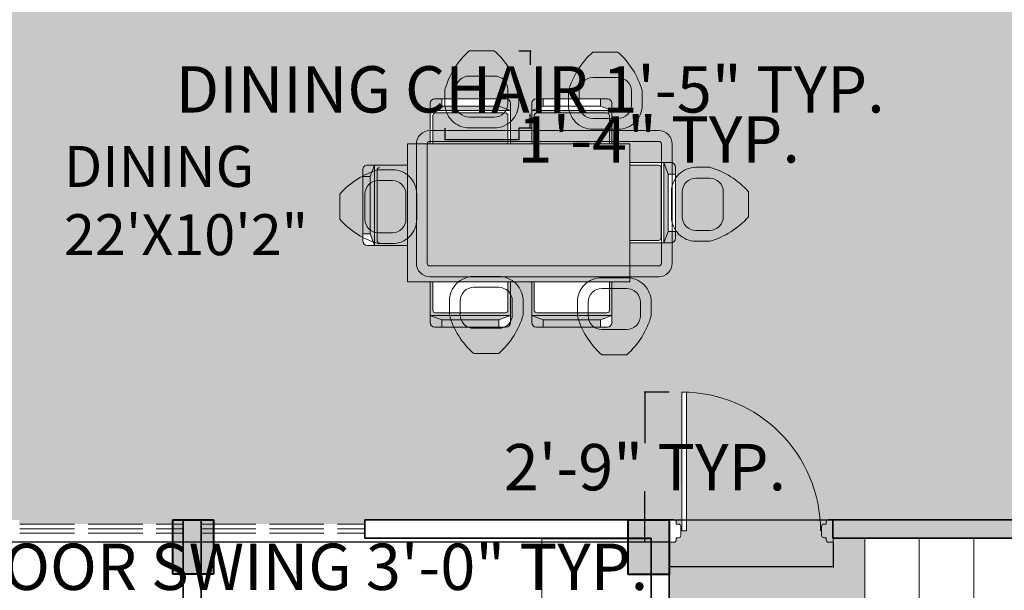
# Model space of a CAD drawing. Units: inches. Extents: x 1077 to 2505, y 1892 to 2728.
# Tile 23 of 26: x 2147 to 2364, y 2298 to 2423. Entities that reach past the tile are written whole.
import ezdxf

# ---------------------------------------------------------------- set-up
doc = ezdxf.new("R2010")
doc.units = ezdxf.units.IN
doc.linetypes.add('ACAD_ISO02W100', pattern=[15, 12, -3])
doc.layers.get('Defpoints').update_dxf_attribs({"color": 220, "linetype": 'ACAD_ISO02W100'})
for name, color, linetype, lineweight in [('00 FURNITURE', 15, 'Continuous', 15), ('A-ANNO-DIMS', 2, 'Continuous', 18), ('A-AREA-IDEN', 7, 'Continuous', 18), ('A-COLS', 7, 'Continuous', 40), ('A-DOOR', 4, 'Continuous', 18), ('A-FLOR-CASE', 8, 'Continuous', 18), ('A-FLOR-STRS', 7, 'Continuous', 18), ('A-GLAZ-OVHD', 160, 'ACAD_ISO02W100', 13), ('A-WALL-PATT', 7, 'Continuous', 9), ('WALL', 7, 'Continuous', 35)]:
    doc.layers.add(name, color=color, linetype=linetype, lineweight=lineweight)
doc.layers.add('A-FLOR-PATT', color=254, linetype='Continuous', lineweight=9, true_color=0xd7ebd2)
doc.styles.get("Standard").update_dxf_attribs({"font": 'arial.ttf'})
doc.dimstyles.get("Standard").update_dxf_attribs({"dimtxt": 10.18, "dimasz": 0.18, "dimexe": 0.18, "dimexo": 0.0625, "dimgap": 0.09, "dimtad": 0, "dimtih": 1, "dimtoh": 1, "dimdec": 0, "dimzin": 0, "dimdsep": 46, "dimlunit": 3, "dimtxsty": 'Standard', "dimcen": 0.09, "dimadec": 0, "dimazin": 0, "dimtfac": 1, "dimtdec": 0, "dimtofl": 0, "dimtmove": 0, "dimatfit": 3, "dimfxl": 1, "dimtolj": 1, "dimtzin": 0, "dimarcsym": 0})

# ---------------------------------------------------------------- blocks, each defined once
blk = doc.blocks.new('DDD')
at = {"layer": '00 FURNITURE'}
for p, q in [((-12579.77, -15859.53), (-12579.77, -15829.05)), ((-12578.77, -15859.53), (-12578.77, -15829.03)), ((-12612.02, -15857.03), (-12612.02, -15862.03)), ((-12611.02, -15857.03), (-12612.02, -15857.03)), ((-12610.52, -15858.03), (-12610.52, -15857.53)), ((-12577.52, -15858.03), (-12577.52, -15857.53)), ((-12577.02, -15857.03), (-12576.02, -15857.03)), ((-12576.02, -15857.03), (-12576.02, -15862.03)), ((-12578.77, -15859.53), (-12579.77, -15859.53)), ((-12612.02, -15862.03), (-12611.02, -15862.03)), ((-12610.52, -15861.53), (-12610.52, -15861.03)), ((-12577.52, -15861.53), (-12577.52, -15861.03)), ((-12576.02, -15862.03), (-12577.02, -15862.03))]:
    blk.add_line(p, q, dxfattribs=at)
for points in [[(-12610.52, -15861.03), (-12610.02, -15861.03, 0.414214), (-12609.52, -15860.53), (-12609.52, -15858.53, 0.414214), (-12610.02, -15858.03), (-12610.52, -15858.03)], [(-12577.52, -15861.03), (-12578.02, -15861.03, -0.414214), (-12578.52, -15860.53), (-12578.52, -15858.53, -0.414214), (-12578.02, -15858.03), (-12577.52, -15858.03)]]:
    blk.add_lwpolyline(points, format="xyb", dxfattribs=at)
for centre, radius, start, end in [((-12578.77, -15859.53), 30.5, 90, 180), ((-12611.02, -15857.53), 0.5, 0, 90), ((-12577.02, -15857.53), 0.5, 90, 180), ((-12611.02, -15861.53), 0.5, 270, 0), ((-12577.02, -15861.53), 0.5, 180, 270)]:
    blk.add_arc(centre, radius, start, end, dxfattribs=at)
blk = doc.blocks.new('C1')
h = blk.add_hatch(color=256)
h.dxf.hatch_style = 1
h.paths.add_polyline_path([(1668.56, 2445.41), (1677.56, 2445.41), (1677.56, 2457.41), (1668.56, 2457.41)])
for p, q in [((1668.56, 2457.41), (1677.56, 2457.41)), ((1668.56, 2445.41), (1668.56, 2457.41)), ((1677.56, 2457.41), (1677.56, 2445.41)), ((1677.56, 2445.41), (1668.56, 2445.41))]:
    blk.add_line(p, q)
blk = doc.blocks.new('DINING-SET-6-SEAT')
for p, q in [((15.87, 50.2), (31.49, 50.2)), ((38.2, 50.2), (53.82, 50.2)), ((14.85, 40.27), (14.85, 49.18)), ((17.38, 48.59), (14.85, 47.63)), ((17.38, 48.59), (29.95, 48.59)), ((29.95, 48.59), (32.51, 47.63)), ((32.51, 49.18), (32.51, 40.27)), ((37.18, 40.27), (37.18, 49.18)), ((39.7, 48.59), (37.18, 47.63)), ((39.7, 48.59), (52.28, 48.59)), ((52.28, 48.59), (54.83, 47.63)), ((54.83, 49.18), (54.83, 40.27)), ((14.85, 47.63), (32.51, 47.63)), ((15.41, 40.27), (15.41, 46.51)), ((15.97, 47.07), (31.38, 47.07)), ((31.94, 46.51), (31.94, 40.27)), ((37.18, 47.63), (54.83, 47.63)), ((37.74, 40.27), (37.74, 46.51)), ((38.3, 47.07), (53.71, 47.07)), ((54.27, 46.51), (54.27, 40.27)), ((58.75, 40.27), (9.82, 40.27)), ((9.82, 9.93), (9.82, 40.27)), ((58.75, 9.93), (58.75, 40.27)), ((9.93, 35.61), (1.02, 35.61)), ((1.62, 33.08), (2.57, 35.61)), ((2.57, 35.61), (2.57, 17.96)), ((58.86, 36.15), (67.76, 36.15)), ((58.86, 35.58), (65.09, 35.58)), ((65.65, 35.02), (65.65, 19.61)), ((67.17, 33.62), (66.22, 36.15)), ((66.22, 36.15), (66.22, 18.49)), ((68.78, 35.13), (68.78, 19.51)), ((0, 34.59), (0, 18.97)), ((1.62, 33.08), (1.62, 20.51)), ((3.13, 34.49), (3.13, 19.08)), ((67.17, 33.62), (67.17, 21.04)), ((1.62, 20.51), (2.57, 17.96)), ((67.17, 21.04), (66.22, 18.49)), ((1.02, 17.96), (9.93, 17.96)), ((65.09, 19.05), (58.86, 19.05)), ((67.76, 18.49), (58.86, 18.49)), ((58.75, 9.93), (9.82, 9.93)), ((14.85, 9.93), (14.85, 1.02)), ((15.41, 9.93), (15.41, 3.69)), ((31.94, 3.69), (31.94, 9.93)), ((32.51, 1.02), (32.51, 9.93)), ((37.18, 9.93), (37.18, 1.02)), ((37.74, 9.93), (37.74, 3.69)), ((54.27, 3.69), (54.27, 9.93)), ((54.83, 1.02), (54.83, 9.93)), ((17.38, 1.61), (14.85, 2.57)), ((14.85, 2.57), (32.51, 2.57)), ((15.97, 3.13), (31.38, 3.13)), ((29.95, 1.61), (32.51, 2.57)), ((39.7, 1.61), (37.18, 2.57)), ((37.18, 2.57), (54.83, 2.57)), ((38.3, 3.13), (53.71, 3.13)), ((52.28, 1.61), (54.83, 2.57)), ((17.38, 1.61), (29.95, 1.61)), ((39.7, 1.61), (52.28, 1.61)), ((15.87, 0), (31.49, 0)), ((38.2, 0), (53.82, 0))]:
    blk.add_line(p, q)
for points in [[(17.38, 50.2), (29.95, 50.2), (29.95, 48.59), (17.38, 48.59)], [(39.7, 50.2), (52.28, 50.2), (52.28, 48.59), (39.7, 48.59)], [(0, 33.08), (0, 20.51), (1.62, 20.51), (1.62, 33.08)], [(68.78, 33.62), (68.78, 21.04), (67.17, 21.04), (67.17, 33.62)], [(17.38, 0), (29.95, 0), (29.95, 1.61), (17.38, 1.61)], [(39.7, 0), (52.28, 0), (52.28, 1.61), (39.7, 1.61)]]:
    blk.add_lwpolyline(points, close=True)
for centre, radius, start, end in [((15.87, 49.18), 1.02, 90.0001, 180.0001), ((31.49, 49.18), 1.02, 0.0001, 90.0001), ((38.2, 49.18), 1.02, 90.0001, 180.0001), ((53.82, 49.18), 1.02, 0.0001, 90.0001), ((15.97, 46.51), 0.56, 90.0001, 180.0001), ((31.38, 46.51), 0.56, 0.0001, 90.0001), ((38.3, 46.51), 0.56, 90.0001, 180.0001), ((53.71, 46.51), 0.56, 0.0001, 90.0001), ((1.02, 34.59), 1.02, 89.9999, 179.9999), ((3.69, 34.49), 0.56, 89.9999, 179.9999), ((65.09, 35.02), 0.56, 0.0001, 90.0001), ((67.76, 35.13), 1.02, 0.0001, 90.0001), ((65.09, 19.61), 0.56, 270.0001, 0.0001), ((67.76, 19.51), 1.02, 270.0001, 0.0001), ((1.02, 18.97), 1.02, 179.9999, 269.9999), ((3.69, 19.08), 0.56, 179.9999, 269.9999), ((15.97, 3.69), 0.56, 179.9999, 269.9999), ((31.38, 3.69), 0.56, 269.9999, 359.9999), ((38.3, 3.69), 0.56, 179.9999, 269.9999), ((53.71, 3.69), 0.56, 269.9999, 359.9999), ((15.87, 1.02), 1.02, 179.9999, 269.9999), ((31.49, 1.02), 1.02, 269.9999, 359.9999), ((38.2, 1.02), 1.02, 179.9999, 269.9999), ((53.82, 1.02), 1.02, 269.9999, 359.9999)]:
    blk.add_arc(centre, radius, start, end)
blk = doc.blocks.new('DINING-CHAIR')
for points in [[(5.36, 16.93), (10.88, 16.93, -0.142909), (16.24, 8.42), (16.24, 5.36, -0.414214), (10.88, 0), (5.36, 0, -0.414214), (0, 5.36), (0, 8.42, -0.142909)], [(5.36, 11.39), (10.88, 11.39, -0.414214), (13.86, 8.42), (13.86, 5.36, -0.414214), (10.88, 2.38), (5.36, 2.38, -0.414214), (2.38, 5.36), (2.38, 8.42, -0.414214)]]:
    blk.add_lwpolyline(points, format="xyb", close=True)
blk = doc.blocks.new('STAIR-PLAN-RETURN')
for p, q in [((0, 163.08), (0, 127.08)), ((12, 163.08), (12, 127.08)), ((24, 163.08), (24, 127.08)), ((36, 163.08), (36, 0)), ((36, 163.08), (36, 127.08)), ((0, 127.08), (72, 127.08)), ((36, 115.08), (72, 115.08)), ((36, 103.08), (72, 103.08)), ((36, 91.08), (72, 91.08)), ((36, 79.08), (72, 79.08)), ((36, 67.08), (72, 67.08)), ((36, 55.08), (72, 55.08)), ((36, 43.08), (72, 43.08)), ((36, 31.08), (72, 31.08)), ((36, 19.08), (72, 19.08)), ((36, 7.08), (72, 7.08)), ((72, 0), (36, 0))]:
    blk.add_line(p, q)
blk = doc.blocks.new('*D46')
at = {"layer": 'A-ANNO-DIMS', "color": 0, "lineweight": -2, "transparency": 16777216}
for p, q in [((2289.89, 2308.17), (2289.89, 2302.65)), ((2325.89, 2308.17), (2325.89, 2302.65)), ((2289.89, 2302.83), (2289.71, 2302.83)), ((2325.71, 2302.83), (2290.07, 2302.83))]:
    blk.add_line(p, q, dxfattribs=at)
at = {"layer": 'A-ANNO-DIMS', "color": 0, "transparency": 16777216}
for points in [[(2290.07, 2302.86), (2290.07, 2302.8), (2289.89, 2302.83)], [(2325.71, 2302.86), (2325.71, 2302.8), (2325.89, 2302.83)]]:
    blk.add_solid(points, dxfattribs=at)
at = {"layer": 'Defpoints', "color": 0, "transparency": 16777216}
for p in [(2289.89, 2308.23), (2325.89, 2308.23), (2289.89, 2302.83)]:
    blk.add_point(p, dxfattribs=at)
at = {"layer": 'A-ANNO-DIMS', "color": 0, "transparency": 16777216, "insert": (2209.47, 2302.83), "char_height": 10.18, "attachment_point": 5}
blk.add_mtext('\\A1;DOOR SWING 3\'-0" TYP.', dxfattribs=at)
blk = doc.blocks.new('*D47')
at = {"layer": 'A-ANNO-DIMS', "color": 0, "lineweight": -2, "transparency": 16777216}
for p, q in [((2289.82, 2341.23), (2284.31, 2341.23)), ((2284.49, 2341.05), (2284.49, 2330.02)), ((2284.49, 2308.41), (2284.49, 2319.44)), ((2289.82, 2308.23), (2284.31, 2308.23))]:
    blk.add_line(p, q, dxfattribs=at)
at = {"layer": 'A-ANNO-DIMS', "color": 0, "transparency": 16777216}
for points in [[(2284.46, 2341.05), (2284.52, 2341.05), (2284.49, 2341.23)], [(2284.46, 2308.41), (2284.52, 2308.41), (2284.49, 2308.23)]]:
    blk.add_solid(points, dxfattribs=at)
at = {"layer": 'Defpoints', "color": 0, "transparency": 16777216}
for p in [(2284.49, 2341.23), (2289.89, 2341.23), (2289.89, 2308.23)]:
    blk.add_point(p, dxfattribs=at)
at = {"layer": 'A-ANNO-DIMS', "color": 0, "transparency": 16777216, "insert": (2284.49, 2324.73), "char_height": 10.18, "attachment_point": 5}
blk.add_mtext('\\A1;2\'-9" TYP.', dxfattribs=at)
blk = doc.blocks.new('*D48')
at = {"layer": 'A-ANNO-DIMS', "color": 0, "lineweight": -2, "transparency": 16777216}
for p, q in [((2256.78, 2416.24), (2259.43, 2416.24)), ((2259.25, 2416.06), (2259.25, 2413.13)), ((2259.25, 2399.49), (2259.25, 2402.42)), ((2256.78, 2399.31), (2259.43, 2399.31))]:
    blk.add_line(p, q, dxfattribs=at)
at = {"layer": 'A-ANNO-DIMS', "color": 0, "transparency": 16777216}
for points in [[(2259.22, 2416.06), (2259.28, 2416.06), (2259.25, 2416.24)], [(2259.22, 2399.49), (2259.28, 2399.49), (2259.25, 2399.31)]]:
    blk.add_solid(points, dxfattribs=at)
at = {"layer": 'Defpoints', "color": 0, "transparency": 16777216}
for p in [(2256.72, 2416.24), (2259.25, 2416.24), (2256.72, 2399.31)]:
    blk.add_point(p, dxfattribs=at)
at = {"layer": 'A-ANNO-DIMS', "color": 0, "transparency": 16777216, "insert": (2259.25, 2407.77), "char_height": 10.18, "attachment_point": 5}
blk.add_mtext('\\A1;DINING CHAIR 1\'-5" TYP.', dxfattribs=at)
blk = doc.blocks.new('*D49')
at = {"layer": 'A-ANNO-DIMS', "color": 0, "lineweight": -2, "transparency": 16777216}
for p, q in [((2240.47, 2399.25), (2240.47, 2396.59)), ((2256.72, 2399.25), (2256.72, 2396.59)), ((2240.65, 2396.77), (2256.54, 2396.77)), ((2256.72, 2396.77), (2256.9, 2396.77))]:
    blk.add_line(p, q, dxfattribs=at)
at = {"layer": 'A-ANNO-DIMS', "color": 0, "transparency": 16777216}
for points in [[(2240.65, 2396.8), (2240.65, 2396.74), (2240.47, 2396.77)], [(2256.54, 2396.8), (2256.54, 2396.74), (2256.72, 2396.77)]]:
    blk.add_solid(points, dxfattribs=at)
at = {"layer": 'Defpoints', "color": 0, "transparency": 16777216}
for p in [(2240.47, 2399.31), (2256.72, 2399.31), (2256.72, 2396.77)]:
    blk.add_point(p, dxfattribs=at)
at = {"layer": 'A-ANNO-DIMS', "color": 0, "transparency": 16777216, "insert": (2287.53, 2396.77), "char_height": 10.18, "attachment_point": 5}
blk.add_mtext('\\A1;1\'-4" TYP.', dxfattribs=at)
blk = doc.blocks.new('*D68')
at = {"layer": 'A-ANNO-DIMS', "color": 0, "lineweight": -2, "transparency": 16777216}
for p, q in [((2289.82, 2308.23), (2006.75, 2308.23)), ((2006.93, 2308.05), (2006.93, 2206.47)), ((2006.93, 2094.32), (2006.93, 2195.9)), ((2289.78, 2094.14), (2006.75, 2094.14))]:
    blk.add_line(p, q, dxfattribs=at)
at = {"layer": 'A-ANNO-DIMS', "color": 0, "transparency": 16777216}
for points in [[(2006.9, 2308.05), (2006.96, 2308.05), (2006.93, 2308.23)], [(2006.9, 2094.32), (2006.96, 2094.32), (2006.93, 2094.14)]]:
    blk.add_solid(points, dxfattribs=at)
at = {"layer": 'Defpoints', "color": 0, "transparency": 16777216}
for p in [(2006.93, 2308.23), (2289.89, 2308.23), (2289.85, 2094.14)]:
    blk.add_point(p, dxfattribs=at)
at = {"layer": 'A-ANNO-DIMS', "color": 0, "transparency": 16777216, "insert": (2006.93, 2201.18), "char_height": 10.18, "attachment_point": 5}
blk.add_mtext('\\A1;17\'-10"', dxfattribs=at)
blk = doc.blocks.new('*D72')
at = {"layer": 'A-ANNO-DIMS', "color": 0, "lineweight": -2, "transparency": 16777216}
for p, q in [((2280.86, 2313.12), (2442.88, 2313.12)), ((2442.7, 2312.94), (2442.7, 2303.7)), ((2442.7, 2283.76), (2442.7, 2292.99)), ((2285.24, 2283.58), (2442.88, 2283.58))]:
    blk.add_line(p, q, dxfattribs=at)
at = {"layer": 'A-ANNO-DIMS', "color": 0, "transparency": 16777216}
for points in [[(2442.67, 2312.94), (2442.73, 2312.94), (2442.7, 2313.12)], [(2442.67, 2283.76), (2442.73, 2283.76), (2442.7, 2283.58)]]:
    blk.add_solid(points, dxfattribs=at)
at = {"layer": 'Defpoints', "color": 0, "transparency": 16777216}
for p in [(2280.8, 2313.12), (2285.18, 2283.58), (2442.7, 2283.58)]:
    blk.add_point(p, dxfattribs=at)
at = {"layer": 'A-ANNO-DIMS', "color": 0, "transparency": 16777216, "insert": (2442.7, 2298.35), "char_height": 10.18, "attachment_point": 5}
blk.add_mtext('\\A1;2\'-5 1/2"', dxfattribs=at)

msp = doc.modelspace()

# ---------------------------------------------------------------- hatches: boundary and pattern name
at = {"layer": 'A-FLOR-PATT', "transparency": 33554559}
h = msp.add_hatch(color=256, dxfattribs=at)
h.dxf.hatch_style = 1
h.paths.add_polyline_path([(2252.85, 2583.14), (2232.15, 2583.14), (2208.15, 2583.17), (2208.15, 2583.14), (2186.85, 2583.14), (2186.85, 2486.14), (2186.85, 2475.14), (2182.85, 2475.14), (2182.85, 2521.11), (2164.84, 2521.11), (2164.84, 2583.14), (2126.63, 2583.14), (2078.63, 2583.13), (2078.63, 2583.14), (2044.85, 2583.14), (2044.85, 2439.14), (2146.85, 2439.14), (2146.85, 2435.14), (2120.85, 2435.14), (2044.85, 2435.14), (2044.85, 2401), (2044.85, 2401), (2044.85, 2377), (2044.85, 2377), (2044.85, 2313.14), (2116.85, 2313.14), (2116.85, 2405.14), (2120.85, 2405.14), (2120.85, 2313.14), (2146.85, 2313.14), (2146.85, 2312.21), (2182.85, 2312.21), (2182.85, 2313.14), (2186.85, 2313.14), (2186.85, 2312.21), (2222.85, 2312.21), (2222.85, 2313.14), (2289.85, 2313.14), (2289.85, 2094.14), (2404.85, 2094.14), (2404.85, 2146.06), (2368.85, 2146.06), (2368.85, 2273.14), (2332.85, 2273.14), (2332.85, 2309.14), (2325.85, 2309.14), (2325.85, 2313.14), (2404.85, 2313.14), (2404.85, 2354.2), (2404.85, 2402.2), (2404.85, 2435.14), (2292.85, 2435.14), (2292.85, 2439.14), (2333.66, 2439.14), (2333.66, 2457.16), (2404.85, 2457.16), (2404.85, 2583.14), (2356.85, 2583.14), (2356.85, 2592.14), (2404.85, 2592.14), (2404.85, 2648.14), (2375.5, 2648.14), (2375.5, 2648.03), (2351.47, 2648.03), (2351.47, 2648.14), (2326.85, 2648.14), (2326.85, 2583.14), (2256.85, 2583.14), (2256.85, 2435.14), (2182.85, 2435.14), (2182.85, 2439.14), (2186.85, 2439.14), (2252.85, 2439.14), (2252.85, 2486.14), (2216.85, 2486.14), (2216.85, 2490.14), (2252.85, 2490.14)])
h.paths.add_polyline_path([(2214.97, 2488.05), (2212.97, 2488.05), (2212.97, 2487.05, 0.414214), (2213.97, 2486.05), (2201.97, 2486.05), (2201.97, 2483.04), (2200.58, 2483.04), (2200.58, 2486.05), (2187.97, 2486.05, -0.414214), (2186.97, 2487.05), (2186.97, 2490.05), (2188.97, 2490.05), (2188.97, 2516.05, -0.446908)], flags=16)
h.paths.add_polyline_path([(2162.4, 2565.16), (2146.2, 2565.16), (2146.2, 2581.36), (2162.4, 2581.36)], flags=16)
h.paths.add_polyline_path([(2161.5, 2566.06), (2147.1, 2566.06), (2147.1, 2580.46), (2161.5, 2580.46)], flags=0)
h.paths.add_polyline_path([(2145.3, 2506.66, -0.414214), (2144.4, 2505.76), (2122.45, 2505.76), (2081.4, 2505.76, -0.414214), (2080.5, 2506.66), (2080.5, 2563.14), (2080.5, 2577.72), (2080.5, 2581.36), (2145.3, 2581.36), (2145.3, 2577.72), (2144.4, 2577.72, -0.414214), (2145.3, 2576.82)], flags=16)
h.paths.add_polyline_path([(2150.3, 2575.03, -1), (2158.24, 2575.03, -1)], flags=0)
h.paths.add_polyline_path([(2150.64, 2575.03, -1), (2157.89, 2575.03, -1)], flags=0)
h.paths.add_polyline_path([(2180.11, 2468.19), (2180.11, 2437.69), (2180.36, 2436.69), (2180.36, 2437.69), (2179.11, 2437.69), (2179.11, 2468.17, 0.404641), (2149.61, 2437.69), (2149.36, 2436.69, -0.414214), (2148.86, 2436.19), (2148.36, 2436.19), (2148.36, 2435.69, -0.414214), (2147.86, 2435.19), (2146.86, 2435.19), (2146.86, 2440.19), (2147.86, 2440.19, -0.414214), (2148.36, 2439.69), (2148.36, 2439.19), (2148.86, 2439.19, -0.414214), (2149.36, 2438.69), (2149.61, 2437.69, -0.414214)], flags=16)
h.paths.add_polyline_path([(2145.14, 2554.26, 0.292232), (2136.49, 2542.78, 0.052719), (2081.25, 2554.26), (2080.6, 2554.26), (2080.6, 2563.14), (2081.25, 2563.14), (2102.73, 2563.14, -0.117785), (2103.09, 2563.91, -0.059418), (2112.19, 2573, -0.379859), (2114.6, 2572.86, -0.02509), (2118.73, 2569.3, -0.025935), (2122.97, 2573, -0.379859), (2125.38, 2572.86, -0.061767), (2134.84, 2563.41, -0.069393), (2135.14, 2563.14), (2145.14, 2563.14)], flags=0)
h.paths.add_polyline_path([(2120.79, 2554.26), (2117.88, 2554.26, -0.015371), (2115.33, 2552.11, -0.429576), (2112.69, 2552.04, -0.016036), (2110.01, 2554.26), (2080.6, 2554.26), (2080.6, 2560.4), (2104.1, 2560.4, 0.055344), (2112.69, 2552.04, 0.331768), (2114.84, 2551.72, 0.027343), (2119.32, 2555.62, 0.00919)], flags=0)
h.paths.add_polyline_path([(2152.88, 2574.32), (2154.19, 2575.07), (2154.19, 2576.58, 0.399698), (2152.71, 2575.03, 0.119004)], flags=0)
h.paths.add_polyline_path([(2152.53, 2575.03, -1), (2156, 2575.03, -1)], flags=0)
h.paths.add_polyline_path([(2154.27, 2574.94), (2154.34, 2574.98), (2154.34, 2575.07), (2154.3, 2575.09), (2154.23, 2574.96)], flags=0)
h.paths.add_polyline_path([(2259.6, 2468.17, -0.414214), (2290.1, 2437.67), (2290.35, 2438.67), (2290.1, 2437.67, 0.404641), (2260.6, 2468.15), (2260.6, 2437.67), (2259.35, 2437.67), (2259.35, 2436.67, -0.414214), (2258.85, 2436.17), (2258.35, 2436.17), (2258.35, 2435.67, -0.414214), (2257.85, 2435.17), (2256.85, 2435.17), (2256.85, 2440.17), (2257.85, 2440.17, -0.414214), (2258.35, 2439.67), (2258.35, 2439.17), (2258.85, 2439.17, -0.414214), (2259.35, 2438.67)], flags=16)
h.paths.add_polyline_path([(2327.48, 2541.19, -0.414214), (2328.38, 2542.09), (2384.85, 2542.09), (2399.43, 2542.09), (2403.08, 2542.09), (2403.08, 2477.29), (2399.43, 2477.29), (2399.43, 2478.19, -0.414214), (2398.53, 2477.29), (2328.38, 2477.29, -0.414214), (2327.48, 2478.19), (2327.48, 2500.14)], flags=16)
h.paths.add_polyline_path([(2340.38, 2542.09, 0.253465), (2337.43, 2532.13, 0.2538), (2327.47, 2529.17)], flags=16)
h.paths.add_polyline_path([(2080.5, 2518.67, 0.253465), (2090.46, 2515.72, 0.2538), (2093.42, 2505.75)], flags=16)
h.paths.add_polyline_path([(2327.09, 2584.7), (2327.09, 2587.7), (2329.09, 2587.7), (2329.09, 2613.7, -0.01951), (2331.09, 2613.66), (2331.09, 2585.7), (2331.09, 2584.7, -0.414214), (2330.09, 2583.7), (2328.09, 2583.7, -0.414214)], flags=16)
h.paths.add_polyline_path([(2239.78, 2404.11), (2252.36, 2404.11), (2252.36, 2405.72), (2239.78, 2405.72)], flags=16)
h.paths.add_polyline_path([(2237.26, 2403.16), (2237.26, 2395.8), (2237.82, 2395.8), (2237.82, 2402.03, -0.41429), (2238.38, 2402.59), (2253.79, 2402.59, -0.414213), (2254.35, 2402.03), (2254.35, 2395.8), (2254.91, 2395.8), (2254.91, 2403.16)], flags=16)
h.paths.add_polyline_path([(2120.69, 2434.12), (2120.69, 2432.12, -0.414214), (2119.69, 2431.12), (2118.69, 2431.12), (2090.73, 2431.12, 0.400854), (2116.69, 2407.02), (2116.69, 2407.12), (2118.69, 2407.12, -0.446908), (2090.69, 2433.12), (2116.69, 2433.12), (2116.69, 2435.12), (2119.69, 2435.12, -0.414214)], flags=16)
h.paths.add_polyline_path([(2262.11, 2404.11), (2274.69, 2404.11), (2274.69, 2405.72), (2262.11, 2405.72)], flags=16)
h.paths.add_polyline_path([(2259.59, 2403.16), (2262.11, 2404.11), (2274.69, 2404.11), (2277.24, 2403.16)], flags=16)
h.paths.add_polyline_path([(2289.58, 2389.14), (2289.58, 2376.57), (2291.19, 2376.57), (2291.19, 2389.14)], flags=16)
h.paths.add_polyline_path([(2288.62, 2391.67), (2281.15, 2391.67), (2281.15, 2391.11), (2287.5, 2391.11, -0.41429), (2288.06, 2390.54), (2288.06, 2375.14, -0.414237), (2287.5, 2374.58), (2281.15, 2374.58), (2281.15, 2374.01), (2288.62, 2374.01)], flags=16)
h.paths.add_polyline_path([(2274.69, 2357.14), (2274.69, 2355.52), (2276.22, 2355.52, 0.414236), (2277.24, 2356.54), (2277.24, 2358.09)], flags=16)
h.paths.add_polyline_path([(2252.36, 2357.14), (2252.36, 2355.52), (2253.89, 2355.52, 0.414235), (2254.91, 2356.54), (2254.91, 2358.09)], flags=16)
h.paths.add_polyline_path([(2224.02, 2376.03), (2222.41, 2376.03), (2222.41, 2374.5, 0.414235), (2223.43, 2373.48), (2224.98, 2373.48)], flags=16)
h.paths.add_polyline_path([(2276.68, 2365.45), (2276.68, 2359.22, -0.41419), (2276.12, 2358.66), (2260.71, 2358.66, -0.414137), (2260.15, 2359.22), (2260.15, 2365.45), (2254.35, 2365.45), (2254.35, 2359.22, -0.414189), (2253.79, 2358.66), (2238.38, 2358.66, -0.414137), (2237.82, 2359.22), (2237.82, 2365.45)], flags=16)
h.paths.add_polyline_path([(2079.6, 2565.16), (2063.4, 2565.16), (2063.4, 2581.36), (2079.6, 2581.36)], flags=16)
h.paths.add_polyline_path([(2078.7, 2566.06), (2064.3, 2566.06), (2064.3, 2580.46), (2078.7, 2580.46)], flags=0)
h.paths.add_polyline_path([(2339.31, 2583.7), (2339.31, 2586.71), (2340.7, 2586.71), (2340.7, 2583.7), (2342.09, 2583.7), (2342.09, 2580.7), (2340.7, 2580.7), (2340.7, 2583.7)], flags=16)
h.paths.add_polyline_path([(2123.69, 2421.51), (2123.69, 2420.12), (2120.69, 2420.12), (2120.69, 2421.51), (2117.68, 2421.51), (2117.68, 2422.89), (2120.69, 2422.89), (2120.69, 2421.51)], flags=16)
h.paths.add_polyline_path([(2067.57, 2575.03, -1), (2075.51, 2575.03, -1)], flags=0)
h.paths.add_polyline_path([(2067.92, 2575.03, -1), (2075.17, 2575.03, -1)], flags=0)
h.paths.add_polyline_path([(2070.16, 2574.32), (2071.47, 2575.07), (2071.47, 2576.58, 0.399698), (2069.99, 2575.03, 0.119004)], flags=0)
h.paths.add_polyline_path([(2069.81, 2575.03, -1), (2073.28, 2575.03, -1)], flags=0)
h.paths.add_polyline_path([(2071.54, 2574.94), (2071.62, 2574.89), (2071.62, 2574.98)], flags=0)
h.paths.add_polyline_path([(2364.5, 2486.1, 0.052719), (2375.98, 2541.34), (2375.98, 2541.99), (2384.85, 2541.99), (2384.85, 2541.34), (2384.85, 2519.86, -0.117785), (2385.62, 2519.51, -0.059418), (2394.72, 2510.41, -0.379859), (2394.58, 2507.99, -0.02509), (2391.01, 2503.87, -0.025935), (2394.72, 2499.62, -0.379859), (2394.58, 2497.21, -0.061767), (2385.12, 2487.75, -0.069393), (2384.85, 2487.45), (2384.85, 2477.45), (2375.98, 2477.45, 0.292232)], flags=0)
h.paths.add_polyline_path([(2373.75, 2509.9, -0.016036), (2375.98, 2512.58), (2375.98, 2541.99), (2382.12, 2541.99), (2382.12, 2518.49, 0.055344), (2373.75, 2509.9, 0.331768), (2373.44, 2507.75, 0.027343), (2377.33, 2503.27, 0.00919), (2375.98, 2501.8), (2375.98, 2504.71, -0.015371), (2373.82, 2507.26, -0.429576)], flags=0)
h.paths.add_polyline_path([(2356.95, 2631.48, -0.171636), (2360.13, 2636.99), (2360.13, 2639.35), (2356, 2639.35, -0.414214), (2355.01, 2640.34), (2355.01, 2646.64, -0.414214), (2356, 2647.62), (2372.14, 2647.62, -0.414214), (2373.13, 2646.64), (2373.13, 2640.34, -0.414214), (2372.14, 2639.35), (2368.01, 2639.35), (2368.01, 2636.99, -0.171636), (2371.2, 2631.48, -0.258205), (2366.63, 2620.45), (2361.51, 2620.45, -0.258205)], flags=16)
h.paths.add_polyline_path([(2358.52, 2631.48, -0.171636), (2361.71, 2636.99), (2366.43, 2636.99, -0.171636), (2369.62, 2631.48, -0.210384), (2366.67, 2622), (2361.47, 2622, -0.210384)], flags=0)
h.paths.add_polyline_path([(2386.88, 2542.99), (2386.88, 2559.19), (2403.08, 2559.19), (2403.08, 2542.99)], flags=16)
h.paths.add_polyline_path([(2387.78, 2543.89), (2387.78, 2558.29), (2402.18, 2558.29), (2402.18, 2543.89)], flags=0)
h.paths.add_polyline_path([(2392.77, 2551.05, -1), (2400.71, 2551.05, -1)], flags=0)
h.paths.add_polyline_path([(2393.11, 2551.05, -1), (2400.37, 2551.05, -1)], flags=0)
h.paths.add_polyline_path([(2386.88, 2476.39), (2403.08, 2476.39), (2403.08, 2460.19), (2386.88, 2460.19)], flags=16)
h.paths.add_polyline_path([(2398.48, 2550.97), (2398.3, 2550.97, -0.544606), (2396.03, 2549.66), (2395.94, 2549.51, 0.547962)], flags=0)
h.paths.add_polyline_path([(2387.78, 2475.49), (2402.18, 2475.49), (2402.18, 2461.09), (2387.78, 2461.09)], flags=0)
h.paths.add_polyline_path([(2396.79, 2551.12), (2396.74, 2551.2), (2396.7, 2551.12)], flags=0)
h.paths.add_polyline_path([(2400.71, 2468.32, -1), (2392.77, 2468.32, -1)], flags=0)
h.paths.add_polyline_path([(2400.37, 2468.32, -1), (2393.11, 2468.32, -1)], flags=0)
h.paths.add_polyline_path([(2398.48, 2468.25), (2398.3, 2468.25, -0.544606), (2396.03, 2466.94), (2395.94, 2466.78, 0.547962)], flags=0)
h.paths.add_polyline_path([(2396.79, 2468.4), (2396.74, 2468.48), (2396.7, 2468.4)], flags=0)
h.paths.add_polyline_path([(2292.64, 2341.23, -0.414214), (2323.14, 2310.73), (2323.39, 2311.73), (2323.14, 2310.73, 0.404641), (2293.64, 2341.21), (2293.64, 2310.73), (2292.39, 2310.73), (2292.39, 2309.73, -0.414214), (2291.89, 2309.23), (2291.39, 2309.23), (2291.39, 2308.73, -0.414214), (2290.89, 2308.23), (2289.89, 2308.23), (2289.89, 2313.23), (2290.89, 2313.23, -0.414214), (2291.39, 2312.73), (2291.39, 2312.23), (2291.89, 2312.23, -0.414214), (2292.39, 2311.73)], flags=16)
h.paths.add_polyline_path([(2389.45, 2641.69), (2392.75, 2641.69), (2392.75, 2641.87), (2389.45, 2641.87)], flags=16)
edge = h.paths.add_edge_path(flags=16)
edge.add_arc((2393.3, 2638.65), 0.183, 270, 360)
edge.add_line((2393.49, 2638.65), (2393.49, 2645.8))
edge.add_line((2393.49, 2645.8), (2395.61, 2645.8))
edge.add_line((2395.61, 2645.8), (2395.61, 2647.8))
edge.add_line((2395.61, 2647.8), (2390.57, 2647.8))
edge.add_line((2390.57, 2647.8), (2390.57, 2645.8))
edge.add_line((2390.57, 2645.8), (2392.19, 2645.8))
edge.add_line((2392.19, 2645.8), (2392.19, 2644.98))
edge.add_line((2392.19, 2644.98), (2391.02, 2644.98))
edge.add_line((2391.02, 2644.98), (2391.02, 2645.8))
edge.add_line((2391.02, 2645.8), (2390.57, 2645.8))
edge.add_line((2390.57, 2645.8), (2390.57, 2647.8))
edge.add_line((2390.57, 2647.8), (2395.61, 2647.8))
edge.add_line((2395.61, 2647.8), (2395.61, 2647.32))
edge.add_line((2395.61, 2647.32), (2397.95, 2647.56))
edge.add_line((2397.95, 2647.56), (2397.95, 2647.8))
edge.add_line((2397.95, 2647.8), (2398.81, 2647.8))
edge.add_line((2398.81, 2647.8), (2398.81, 2647.23))
edge.add_line((2398.81, 2647.23), (2398.63, 2645.77))
edge.add_ellipse((2398.41, 2644.93), major_axis=(-1.08, 0), ratio=0.790849, start_angle=180, end_angle=255.2976, ccw=False)
edge.add_line((2399.49, 2644.93), (2399.49, 2644.36))
edge.add_ellipse((2398.41, 2644.36), major_axis=(-1.08, 0), ratio=0.790849, start_angle=0, end_angle=180, ccw=False)
edge.add_line((2397.32, 2644.36), (2397.33, 2644.85))
edge.add_ellipse((2398.41, 2644.93), major_axis=(-1.08, 0), ratio=0.790849, start_angle=284.7024, end_angle=364.0401, ccw=False)
edge.add_line((2398.1, 2645.73), (2398.1, 2647.23))
edge.add_line((2398.1, 2647.23), (2397.95, 2647.23))
edge.add_line((2397.95, 2647.23), (2395.61, 2646.99))
edge.add_line((2395.61, 2646.99), (2395.61, 2645.8))
edge.add_line((2395.61, 2645.8), (2393.49, 2645.8))
edge.add_line((2393.49, 2645.8), (2393.49, 2638.46))
edge.add_line((2393.49, 2638.46), (2393.3, 2638.46))
h.paths.add_polyline_path([(2353.64, 2256.32, -0.292371), (2356.22, 2253.81, -0.085148), (2358.52, 2214.83, -0.01331), (2357.59, 2104.48, -0.379287), (2354.54, 2101.26, -0.0502), (2298.86, 2101.26, -0.379287), (2295.81, 2104.48, -0.01331), (2294.88, 2214.83, -0.086132), (2297.28, 2254.24, -0.295116), (2299.9, 2256.76, -0.114238)], flags=16)
h.paths.add_polyline_path([(2352.48, 2211.82, -0.355389), (2354.02, 2208.08), (2350.26, 2195.63, -0.398275), (2346.44, 2193.45, 0.113332), (2306.96, 2193.45, -0.398275), (2303.14, 2195.63), (2299.38, 2208.08, -0.355394), (2300.92, 2211.82, -0.265725)], flags=0)
h.paths.add_polyline_path([(2297.68, 2201.7), (2303.26, 2187.65), (2303.26, 2166.61), (2298.16, 2163.24)], flags=0)
h.paths.add_polyline_path([(2355.78, 2201.7), (2355.31, 2163.24), (2350.2, 2166.61), (2350.2, 2187.65)], flags=0)
h.paths.add_polyline_path([(2303.26, 2164.35), (2303.26, 2143.1), (2298.44, 2128.54), (2298.19, 2161.01)], flags=0)
h.paths.add_polyline_path([(2350.2, 2164.35), (2355.28, 2161.01), (2355.03, 2128.54), (2350.2, 2143.1)], flags=0)
h.paths.add_polyline_path([(2347.2, 2136.38), (2351.71, 2113.65, -0.090102), (2301.76, 2113.63), (2306.27, 2136.37, 0.036636)], flags=0)
h.paths.add_polyline_path([(2304.86, 2165.32), (2354.76, 2165.32), (2354.76, 2183.87), (2304.86, 2183.87)], flags=8)
h.paths.add_polyline_path([(2053.76, 2360.82), (2103.97, 2360.82), (2103.97, 2394.41), (2053.76, 2394.41)], flags=24)
h.paths.add_polyline_path([(2153.41, 2366.23), (2211.12, 2366.23), (2211.12, 2399.82), (2153.41, 2399.82)], flags=24)
h.paths.add_polyline_path([(2258.04, 2477.83), (2327.95, 2477.83), (2327.95, 2511.42), (2258.04, 2511.42)], flags=24)
h.paths.add_polyline_path([(2182.1, 2454.46), (2252.27, 2454.46), (2252.27, 2473), (2182.1, 2473)], flags=24)
h.paths.add_polyline_path([(2192.4, 2537.41), (2246.99, 2537.41), (2246.99, 2571), (2192.4, 2571)], flags=24)
h.paths.add_polyline_path([(2083.07, 2465.98), (2152.99, 2465.98), (2152.99, 2499.56), (2083.07, 2499.56)], flags=24)
at = {"layer": 'A-WALL-PATT', "transparency": 33554585}
h = msp.add_hatch(color=256, dxfattribs=at)
h.dxf.hatch_style = 1
h.paths.add_polyline_path([(2044.85, 2429.98), (2035.85, 2429.98), (2035.85, 2401), (2044.85, 2401)])
h.paths.add_polyline_path([(2044.85, 2377), (2035.85, 2377), (2035.85, 2317.47), (2044.85, 2317.47)])
h.paths.add_polyline_path([(2085.45, 2159.14), (2044.85, 2159.14), (2044.85, 2225.64), (2035.85, 2225.64), (2035.85, 2106.16), (2044.85, 2106.16), (2044.85, 2150.14), (2085.45, 2150.14)])
h.paths.add_polyline_path([(2289.85, 2103.14), (2044.85, 2103.14), (2044.85, 2106.16), (2035.85, 2106.16), (2035.85, 2094.14), (2289.85, 2094.14)])
h.paths.add_polyline_path([(2413.85, 2354.2), (2404.85, 2354.2), (2404.85, 2354.2), (2404.85, 2313.14), (2325.85, 2313.14), (2325.85, 2309.14), (2404.85, 2309.14), (2404.85, 2094.14), (2413.85, 2094.14)])
h.paths.add_polyline_path([(2413.85, 2431.09), (2404.85, 2431.09), (2404.85, 2402.2), (2413.85, 2402.2)])
h.paths.add_polyline_path([(2404.85, 2439.14), (2292.85, 2439.14), (2292.85, 2435.14), (2404.85, 2435.14)])
h.paths.add_polyline_path([(2413.85, 2580.36), (2404.85, 2580.36), (2404.85, 2457.16), (2404.87, 2457.16), (2404.87, 2443.09), (2413.85, 2443.09)])
h.paths.add_polyline_path([(2413.85, 2645.09), (2404.85, 2645.09), (2404.85, 2592.36), (2413.85, 2592.36)])
h.paths.add_polyline_path([(2413.85, 2645.09), (2404.85, 2645.09), (2404.85, 2648.14), (2375.5, 2648.14), (2375.5, 2648.03), (2351.5, 2648.03), (2351.5, 2657.03), (2375.47, 2657.03), (2375.47, 2657.14), (2413.85, 2657.14)])
h.paths.add_polyline_path([(2351.47, 2657.14), (2326.92, 2657.14), (2326.92, 2648.14), (2351.47, 2648.14)])
h.paths.add_polyline_path([(2078.63, 2583.14), (2044.92, 2583.14), (2044.92, 2580.01), (2035.92, 2580.01), (2035.92, 2592.14), (2078.63, 2592.14)])
h.paths.add_polyline_path([(2180.39, 2592.14), (2126.63, 2592.14), (2126.63, 2583.14), (2180.39, 2583.14)])
h.paths.add_polyline_path([(2232.16, 2592.17), (2232.16, 2583.17), (2208.16, 2583.17), (2208.15, 2583.17), (2208.15, 2583.14), (2189.39, 2583.14), (2189.39, 2579.98), (2180.39, 2579.98), (2180.39, 2592.14), (2208.15, 2592.14), (2208.16, 2592.14), (2208.16, 2592.17)])
h.paths.add_polyline_path([(2250.27, 2592.14), (2232.16, 2592.14), (2232.16, 2583.14), (2250.27, 2583.14)], flags=17)
h.paths.add_polyline_path([(2326.85, 2648.14), (2326.92, 2657.14), (2317.85, 2657.14), (2317.85, 2592.14), (2250.27, 2592.14), (2250.27, 2583.14), (2252.85, 2583.14), (2252.85, 2490.14), (2216.85, 2490.14), (2216.85, 2486.14), (2252.85, 2486.14), (2252.85, 2439.14), (2186.85, 2439.14), (2182.85, 2439.14), (2182.85, 2435.14), (2256.85, 2435.14), (2256.85, 2583.14), (2326.85, 2583.14)])
h.paths.add_polyline_path([(2044.85, 2580.01), (2035.85, 2580.01), (2035.85, 2441.98), (2044.85, 2441.98)])

# ---------------------------------------------------------------- linework, layer by layer
at = {"layer": '00 FURNITURE'}
for points in [[(2237.17, 2398.73), (2287.52, 2398.73, -0.414214), (2290.5, 2395.76), (2290.5, 2369.56, -0.414214), (2287.52, 2366.59), (2237.17, 2366.59, -0.414214), (2234.2, 2369.56), (2234.2, 2395.76, -0.414214)], [(2237.17, 2396.35), (2287.52, 2396.35, -0.414214), (2288.12, 2395.76), (2288.12, 2369.56, -0.414214), (2287.52, 2368.97), (2237.17, 2368.97, -0.414214), (2236.58, 2369.56), (2236.58, 2395.76, -0.414214)]]:
    msp.add_lwpolyline(points, format="xyb", close=True, dxfattribs=at)
at = {"layer": 'A-FLOR-CASE'}
for p, q in [((2285.78, 2308.99), (2261.78, 2308.99)), ((2261.78, 2308.99), (2261.78, 2227.18))]:
    msp.add_line(p, q, dxfattribs=at)
at = {"layer": 'A-GLAZ-OVHD'}
for p, q in [((2146.97, 2312.21), (2182.85, 2312.21)), ((2186.85, 2312.21), (2222.85, 2312.21)), ((2146.97, 2311.21), (2182.85, 2311.21)), ((2146.97, 2310.21), (2182.85, 2310.21)), ((2186.85, 2311.21), (2222.85, 2311.21)), ((2186.85, 2310.21), (2222.85, 2310.21))]:
    msp.add_line(p, q, dxfattribs=at)
at = {"layer": 'WALL'}
for p, q in [((2182.85, 2313.14), (2186.85, 2313.14)), ((2182.85, 2195.14), (2182.85, 2313.14)), ((2186.85, 2203.14), (2186.85, 2313.14)), ((2222.85, 2313.14), (2289.85, 2313.14)), ((2222.85, 2309.14), (2222.85, 2313.14)), ((2289.85, 2094.14), (2289.85, 2313.14)), ((2325.85, 2313.14), (2404.85, 2313.14)), ((2325.85, 2309.14), (2325.85, 2313.14)), ((2222.85, 2309.14), (2285.85, 2309.14)), ((2285.85, 2203.14), (2285.85, 2309.14)), ((2325.85, 2309.14), (2404.85, 2309.14))]:
    msp.add_line(p, q, dxfattribs=at)

# ---------------------------------------------------------------- block references
at = {"layer": '00 FURNITURE'}
for name, p in [('DINING-CHAIR', (2240.47, 2399.31)), ('DINING-CHAIR', (2267.67, 2399.01)), ('DINING-SET-6-SEAT', (2222.41, 2355.52))]:
    msp.add_blockref(name, p, dxfattribs=at)
at = {"layer": '00 FURNITURE', "rotation": 89.99999999999994}
msp.add_blockref('DINING-CHAIR', (2234.28, 2373.87), dxfattribs=at)
at = {"layer": '00 FURNITURE', "extrusion": (0, 0, -1), "zscale": -1}
for p, rotation in [((-2290.34, 2374.4), 89.99999999999973), ((-2241.45, 2366.64), 180), ((-2269.62, 2366.38), 180)]:
    msp.add_blockref('DINING-CHAIR', p, dxfattribs=dict(at, rotation=rotation))
at = {"layer": 'A-COLS'}
for p in [(512.02, -144.22), (612.24, -144.29)]:
    msp.add_blockref('C1', p, dxfattribs=at)
at = {"layer": 'A-DOOR', "xscale": -1}
msp.add_blockref('DDD', (-10286.14, 18170.26), dxfattribs=at)
at = {"layer": 'A-FLOR-STRS'}
msp.add_blockref('STAIR-PLAN-RETURN', (2332.85, 2146.06), dxfattribs=at)

# ---------------------------------------------------------------- texts
at = {"layer": 'A-AREA-IDEN', "insert": (2156.63, 2395.34), "char_height": 9, "attachment_point": 1}
msp.add_mtext_dynamic_manual_height_columns('DINING\\P22\'X10\'2"', width=128.1076, gutter_width=12.5, heights=[0], dxfattribs=at)

# ---------------------------------------------------------------- dimensions: what is measured, and where the dimension line sits
at = {"layer": 'A-ANNO-DIMS'}
for base, p1, p2, angle, text, picture, middle in [((2259.25, 2416.24), (2256.72, 2399.31), (2256.72, 2416.24), 90, 'DINING CHAIR <> TYP.', '*D48', (2259.25, 2407.77)), ((2284.49, 2341.23), (2289.89, 2308.23), (2289.89, 2341.23), 90, '<> TYP.', '*D47', (2284.49, 2324.73)), ((2289.89, 2302.83), (2325.89, 2308.23), (2289.89, 2308.23), 180, 'DOOR SWING <> TYP.', '*D46', (2209.47, 2302.83))]:
    dim = msp.add_linear_dim(base=base, p1=p1, p2=p2, angle=angle, text=text, dimstyle='Standard', override={"dimdec": 1, "dimlfac": 1, "dimrnd": 0, "dimzin": 1, "dimdsep": 46, "dimlunit": 4, "dimfrac": 2}, dxfattribs=at)
    dim.commit()
    dim.dimension.update_dxf_attribs({"geometry": picture, "text_midpoint": middle})
dim = msp.add_linear_dim(base=(2256.7153, 2396.7711), p1=(2240.472, 2399.3101), p2=(2256.7153, 2399.3101), text='<> TYP.', dimstyle='Standard', override={"dimdec": 1, "dimlfac": 1, "dimrnd": 0, "dimzin": 1, "dimdsep": 46, "dimlunit": 4, "dimfrac": 2}, dxfattribs=at)
dim.commit()
dim.dimension.update_dxf_attribs({"geometry": '*D49', "text_midpoint": (2287.5323, 2396.7711)})
for base, p1, p2, picture, middle in [((2442.7, 2283.58), (2280.8, 2313.12), (2285.18, 2283.58), '*D72', (2442.7, 2298.35)), ((2006.93, 2308.23), (2289.85, 2094.14), (2289.89, 2308.23), '*D68', (2006.93, 2201.18))]:
    dim = msp.add_linear_dim(base=base, p1=p1, p2=p2, angle=90, dimstyle='Standard', override={"dimdec": 1, "dimlfac": 1, "dimrnd": 0, "dimzin": 1, "dimdsep": 46, "dimlunit": 4, "dimfrac": 2}, dxfattribs=at)
    dim.commit()
    dim.dimension.update_dxf_attribs({"geometry": picture, "text_midpoint": middle})

doc.saveas('drawing.dxf')
